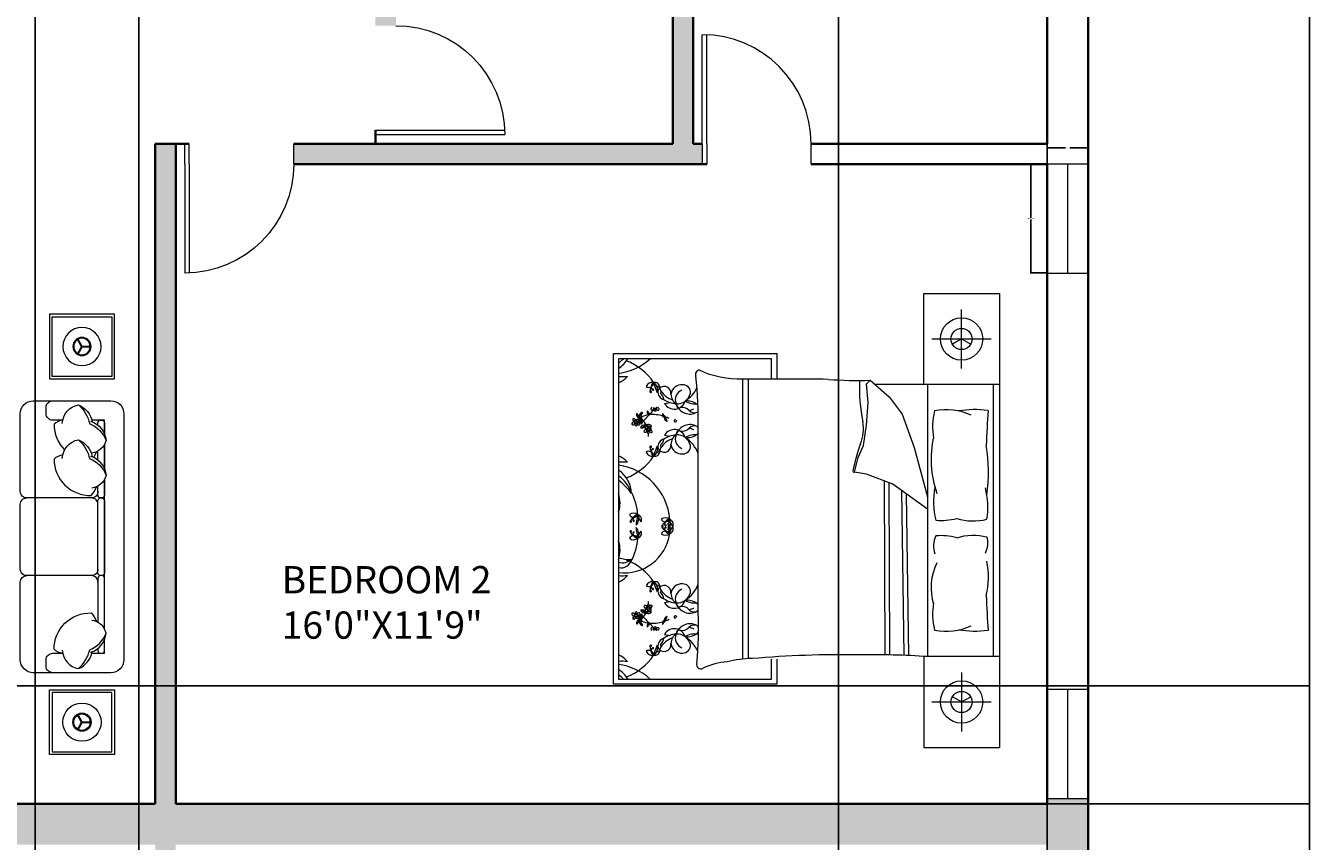
# Model space of a CAD drawing. Units: inches. Extents: x -26 to 13070, y -956 to 6917.
# Tile 9 of 13: x 314 to 597, y -466 to -286. Entities that reach past the tile are written whole.
import ezdxf

# ---------------------------------------------------------------- set-up
doc = ezdxf.new("R2010")
doc.units = ezdxf.units.IN
doc.header["$MEASUREMENT"] = 0
for name, color, linetype, lineweight in [('A-ANNO-DIMS', 2, 'Continuous', 18), ('A-AREA-IDEN', 7, 'Continuous', 18), ('A-DOOR', 3, 'Continuous', 18), ('A-FURN', 8, 'Continuous', 13), ('A-GLAZ', 4, 'Continuous', 18), ('A-WALL', 7, 'Continuous', 35), ('A-WALL-PATT', 252, 'Continuous', 13)]:
    doc.layers.add(name, color=color, linetype=linetype, lineweight=lineweight)
doc.styles.get("Standard").update_dxf_attribs({"font": 'arial.ttf'})
doc.dimstyles.get("Standard").update_dxf_attribs({"dimtxt": 0.18, "dimasz": 0.18, "dimexe": 0.18, "dimexo": 0.0625, "dimgap": 0.09, "dimtad": 0, "dimtih": 1, "dimtoh": 1, "dimdec": 0, "dimzin": 0, "dimdsep": 46, "dimlunit": 3, "dimtxsty": 'Standard', "dimcen": 0.09, "dimadec": 0, "dimazin": 0, "dimtfac": 1, "dimtdec": 0, "dimtofl": 0, "dimtmove": 0, "dimatfit": 3, "dimfxl": 1, "dimtolj": 1, "dimtzin": 0, "dimarcsym": 0})

# ---------------------------------------------------------------- blocks, each defined once
blk = doc.blocks.new('LIVING-END-TABLE')
for p, q in [((7.06, 7.09), (6.05, 8.83)), ((7.21, 7.18), (6.21, 8.92)), ((7.06, 7.18), (6.05, 5.44)), ((7.21, 7.09), (6.21, 5.35)), ((7.13, 7.22), (9.15, 7.22)), ((7.13, 7.04), (9.15, 7.04))]:
    blk.add_line(p, q)
at = {"ltscale": 0.03}
blk.add_lwpolyline([(0, 0), (0, 14.27), (14.27, 14.27), (14.27, 0)], close=True, dxfattribs=at)
blk.add_lwpolyline([(0.57, 13.7), (0.57, 0.57), (13.7, 0.57), (13.7, 13.7)], close=True)
for radius in [4.21, 2.01, 1.81]:
    blk.add_circle((7.13, 7.13), radius)
blk = doc.blocks.new('DOOR-SWING-24')
for p, q in [((24, 1), (0, 1)), ((24, 0), (0, 0))]:
    blk.add_line(p, q)
blk.add_arc((24, 0), 24, 90, 180)
blk = doc.blocks.new('WIN-24')
for p, q in [((0, 24), (0, 0)), ((9, 24), (0, 24)), ((4.5, 24), (4.5, 0)), ((9, 0), (9, 24)), ((0, 0), (9, 0))]:
    blk.add_line(p, q)
blk = doc.blocks.new('*D22')
at = {"layer": 'A-ANNO-DIMS', "color": 0, "lineweight": -2, "transparency": 16777216}
for p, q in [((538.58, -316.54), (534.86, -316.54)), ((535.04, -316.72), (535.04, -328.36)), ((535.04, -340.36), (535.04, -328.72)), ((538.58, -340.54), (534.86, -340.54))]:
    blk.add_line(p, q, dxfattribs=at)
at = {"layer": 'A-ANNO-DIMS', "color": 0, "transparency": 16777216}
for points in [[(535.01, -316.72), (535.07, -316.72), (535.04, -316.54)], [(535.01, -340.36), (535.07, -340.36), (535.04, -340.54)]]:
    blk.add_solid(points, dxfattribs=at)
at = {"layer": 'Defpoints', "color": 0, "transparency": 16777216}
for p in [(535.04, -316.54), (538.64, -316.54), (538.64, -340.54)]:
    blk.add_point(p, dxfattribs=at)
at = {"layer": 'A-ANNO-DIMS', "color": 0, "transparency": 16777216, "insert": (535.04, -328.54), "char_height": 0.18, "attachment_point": 5}
blk.add_mtext('\\A1;WINDOW 24 TYP.', dxfattribs=at)
blk = doc.blocks.new('*D23')
at = {"layer": 'A-ANNO-DIMS', "color": 0, "lineweight": -2, "transparency": 16777216}
for p, q in [((538.64, -316.48), (538.64, -312.76)), ((538.82, -312.94), (542.68, -312.94)), ((547.46, -312.94), (543.6, -312.94)), ((547.64, -316.48), (547.64, -312.76))]:
    blk.add_line(p, q, dxfattribs=at)
at = {"layer": 'A-ANNO-DIMS', "color": 0, "transparency": 16777216}
for points in [[(538.82, -312.91), (538.82, -312.97), (538.64, -312.94)], [(547.46, -312.91), (547.46, -312.97), (547.64, -312.94)]]:
    blk.add_solid(points, dxfattribs=at)
at = {"layer": 'Defpoints', "color": 0, "transparency": 16777216}
for p in [(547.64, -312.94), (538.64, -316.54), (547.64, -316.54)]:
    blk.add_point(p, dxfattribs=at)
at = {"layer": 'A-ANNO-DIMS', "color": 0, "transparency": 16777216, "insert": (543.14, -312.94), "char_height": 0.18, "attachment_point": 5}
blk.add_mtext('\\A1;9 TYP.', dxfattribs=at)
blk = doc.blocks.new('*D45')
at = {"layer": 'A-ANNO-DIMS', "color": 0, "lineweight": -2, "transparency": 16777216}
for p, q in [((547.7, 10.46), (596.57, 10.46)), ((596.39, 10.28), (596.39, -223.36)), ((596.39, -457.36), (596.39, -223.72)), ((538.7, -457.54), (596.57, -457.54))]:
    blk.add_line(p, q, dxfattribs=at)
at = {"layer": 'A-ANNO-DIMS', "color": 0, "transparency": 16777216}
for points in [[(596.36, 10.28), (596.42, 10.28), (596.39, 10.46)], [(596.36, -457.36), (596.42, -457.36), (596.39, -457.54)]]:
    blk.add_solid(points, dxfattribs=at)
at = {"layer": 'Defpoints', "color": 0, "transparency": 16777216}
for p in [(547.64, 10.46), (596.39, 10.46), (538.64, -457.54)]:
    blk.add_point(p, dxfattribs=at)
at = {"layer": 'A-ANNO-DIMS', "color": 0, "transparency": 16777216, "insert": (596.39, -223.54), "char_height": 0.18, "attachment_point": 5}
blk.add_mtext('\\A1;468', dxfattribs=at)
blk = doc.blocks.new('*D46')
at = {"layer": 'A-ANNO-DIMS', "color": 0, "lineweight": -2, "transparency": 16777216}
for p, q in [((538.7, -457.54), (596.57, -457.54)), ((596.39, -457.72), (596.39, -665.86)), ((596.39, -874.36), (596.39, -666.22)), ((547.7, -874.54), (596.57, -874.54))]:
    blk.add_line(p, q, dxfattribs=at)
at = {"layer": 'A-ANNO-DIMS', "color": 0, "transparency": 16777216}
for points in [[(596.36, -457.72), (596.42, -457.72), (596.39, -457.54)], [(596.36, -874.36), (596.42, -874.36), (596.39, -874.54)]]:
    blk.add_solid(points, dxfattribs=at)
at = {"layer": 'Defpoints', "color": 0, "transparency": 16777216}
for p in [(538.64, -457.54), (596.39, -457.54), (547.64, -874.54)]:
    blk.add_point(p, dxfattribs=at)
at = {"layer": 'A-ANNO-DIMS', "color": 0, "transparency": 16777216, "insert": (596.39, -666.04), "char_height": 0.18, "attachment_point": 5}
blk.add_mtext('\\A1;417', dxfattribs=at)
blk = doc.blocks.new('*D50')
at = {"layer": 'A-ANNO-DIMS', "color": 0, "lineweight": -2, "transparency": 16777216}
for p, q in [((315.7, -495.61), (315.7, 116.39)), ((315.88, 116.21), (326.72, 116.21)), ((338.35, 116.21), (327.51, 116.21)), ((338.53, -495.61), (338.53, 116.39))]:
    blk.add_line(p, q, dxfattribs=at)
at = {"layer": 'A-ANNO-DIMS', "color": 0, "transparency": 16777216}
for points in [[(315.88, 116.24), (315.88, 116.18), (315.7, 116.21)], [(338.35, 116.24), (338.35, 116.18), (338.53, 116.21)]]:
    blk.add_solid(points, dxfattribs=at)
at = {"layer": 'Defpoints', "color": 0, "transparency": 16777216}
for p in [(338.53, 116.21), (315.7, -495.67), (338.53, -495.67)]:
    blk.add_point(p, dxfattribs=at)
at = {"layer": 'A-ANNO-DIMS', "color": 0, "transparency": 16777216, "insert": (327.12, 116.21), "char_height": 0.18, "attachment_point": 5}
blk.add_mtext('\\A1;22.83', dxfattribs=at)
blk = doc.blocks.new('*D53')
at = {"layer": 'A-ANNO-DIMS', "color": 0, "lineweight": -2, "transparency": 16777216}
for p, q in [((492.64, -622.48), (492.64, 116.39)), ((492.82, 116.21), (515.42, 116.21)), ((538.46, 116.21), (515.86, 116.21)), ((538.64, -622.48), (538.64, 116.39))]:
    blk.add_line(p, q, dxfattribs=at)
at = {"layer": 'A-ANNO-DIMS', "color": 0, "transparency": 16777216}
for points in [[(492.82, 116.24), (492.82, 116.18), (492.64, 116.21)], [(538.46, 116.24), (538.46, 116.18), (538.64, 116.21)]]:
    blk.add_solid(points, dxfattribs=at)
at = {"layer": 'Defpoints', "color": 0, "transparency": 16777216}
for p in [(538.64, 116.21), (492.64, -622.54), (538.64, -622.54)]:
    blk.add_point(p, dxfattribs=at)
at = {"layer": 'A-ANNO-DIMS', "color": 0, "transparency": 16777216, "insert": (515.64, 116.21), "char_height": 0.18, "attachment_point": 5}
blk.add_mtext('\\A1;46', dxfattribs=at)
blk = doc.blocks.new('*D57')
at = {"layer": 'A-ANNO-DIMS', "color": 0, "lineweight": -2, "transparency": 16777216}
for p, q in [((154.7, -271.54), (596.57, -271.54)), ((596.39, -271.72), (596.39, -351.36)), ((596.39, -431.36), (596.39, -351.72)), ((154.7, -431.54), (596.57, -431.54))]:
    blk.add_line(p, q, dxfattribs=at)
at = {"layer": 'A-ANNO-DIMS', "color": 0, "transparency": 16777216}
for points in [[(596.36, -271.72), (596.42, -271.72), (596.39, -271.54)], [(596.36, -431.36), (596.42, -431.36), (596.39, -431.54)]]:
    blk.add_solid(points, dxfattribs=at)
at = {"layer": 'Defpoints', "color": 0, "transparency": 16777216}
for p in [(154.64, -271.54), (596.39, -271.54), (154.64, -431.54)]:
    blk.add_point(p, dxfattribs=at)
at = {"layer": 'A-ANNO-DIMS', "color": 0, "transparency": 16777216, "insert": (596.39, -351.54), "char_height": 0.18, "attachment_point": 5}
blk.add_mtext('\\A1;160', dxfattribs=at)

msp = doc.modelspace()

# ---------------------------------------------------------------- hatches: boundary and pattern name
at = {"layer": 'A-WALL-PATT'}
h = msp.add_hatch(color=256, dxfattribs=at)
h.dxf.hatch_style = 1
h.paths.add_polyline_path([(223.641, 10.458), (214.641, 10.458), (22.641, 10.458), (22.641, -171.042), (31.641, -171.042), (31.641, -135.042), (205.641, -135.042), (205.641, -241.042), (210.141, -241.042), (210.141, -130.542), (94.641, -130.542), (94.641, -76.542), (85.641, -76.542), (85.641, -126.042), (27.141, -126.042), (27.141, 5.958), (85.641, 5.958), (85.641, -52.542), (94.641, -52.542), (94.641, 1.458), (214.641, 1.458), (214.641, -16.542), (223.641, -16.542), (229.641, -16.542), (229.641, -7.542), (223.641, -7.542)])
h.paths.add_polyline_path([(367.048, 10.458), (346.641, 10.458), (337.641, 10.458), (337.641, -7.542), (331.641, -7.542), (331.641, -16.542), (337.641, -16.542), (342.141, -16.542), (342.141, -128.542), (346.641, -128.542), (346.641, 1.458), (367.048, 1.458)])
h.paths.add_polyline_path([(547.641, 10.458), (403.048, 10.458), (403.048, 1.458), (538.641, 1.458), (538.641, -46.542), (547.641, -46.542)])
h.paths.add_polyline_path([(547.641, -106.542), (538.641, -106.542), (538.641, -154.542), (481.013, -154.542), (481.013, -159.042), (538.641, -159.042), (547.641, -159.042)])
h.paths.add_polyline_path([(457.013, -154.542), (342.141, -154.542), (342.141, -165.042), (346.641, -165.042), (346.641, -159.042), (414.141, -159.042), (414.141, -225.042), (346.641, -225.042), (346.641, -189.042), (342.141, -189.042), (342.141, -234.042), (390.641, -234.042), (390.641, -286.042), (395.141, -286.042), (395.141, -234.042), (456.141, -234.042), (456.141, -312.042), (372.641, -312.042), (372.641, -316.542), (462.641, -316.542), (462.641, -312.042), (460.641, -312.042), (460.641, -234.042), (538.641, -234.042), (547.641, -234.042), (547.641, -195.042), (538.641, -195.042), (538.641, -225.042), (418.641, -225.042), (418.641, -159.042), (457.013, -159.042)])
h.paths.add_polyline_path([(547.641, -270.042), (538.641, -270.042), (538.641, -312.042), (486.641, -312.042), (486.641, -316.542), (538.641, -316.542), (547.641, -316.542)], flags=0)
h.paths.add_polyline_path([(547.641, -456.306), (538.641, -456.306), (538.641, -457.542), (346.641, -457.542), (346.641, -316.542), (346.641, -312.042), (342.141, -312.042), (342.141, -457.542), (145.641, -457.542), (145.641, -466.542), (342.141, -466.542), (342.141, -627.042), (346.641, -627.042), (346.641, -466.542), (538.641, -466.542), (538.641, -514.542), (547.641, -514.542)])
h.paths.add_polyline_path([(466.641, -622.542), (372.641, -622.542), (372.641, -627.042), (388.641, -627.042), (388.641, -721.542), (393.141, -721.542), (393.141, -627.042), (462.141, -627.042), (462.141, -717.042), (466.641, -717.042)])
h.paths.add_polyline_path([(547.641, -574.542), (538.641, -574.542), (538.641, -622.542), (492.641, -622.542), (492.641, -627.042), (538.641, -627.042), (538.641, -654.042), (547.641, -654.042)])
h.paths.add_polyline_path([(547.641, -690.042), (538.641, -690.042), (538.641, -717.042), (466.641, -717.042), (466.641, -721.542), (538.641, -721.542), (538.641, -763.542), (547.641, -763.542)])
h.paths.add_polyline_path([(462.141, -717.042), (419.141, -717.042), (419.141, -721.542), (462.141, -721.542)], flags=0)
h.paths.add_polyline_path([(346.641, -721.542), (352.641, -721.542), (352.641, -717.042), (342.141, -717.042), (342.141, -874.542), (342.141, -907.542), (351.141, -907.542), (351.141, -874.542), (395.949, -874.542), (395.949, -865.542), (351.141, -865.542), (351.141, -841.542), (346.641, -841.542)])
h.paths.add_polyline_path([(547.641, -823.542), (538.641, -823.542), (538.641, -865.542), (431.949, -865.542), (431.949, -874.542), (547.641, -874.542)])
h.paths.add_polyline_path([(172.641, -865.713), (140.641, -865.744), (140.641, -788.744), (182.646, -788.704), (182.641, -784.204), (136.141, -784.249), (136.141, -848.332), (131.641, -848.332), (131.641, -874.542), (172.641, -874.542)])
h.paths.add_polyline_path([(217.641, -816.13), (213.141, -816.13), (213.141, -784.174), (208.641, -784.179), (208.641, -865.679), (208.641, -874.542), (217.641, -874.542)])
h.paths.add_polyline_path([(95.641, -865.788), (31.641, -865.849), (31.641, -832.695), (22.641, -832.695), (22.641, -874.542), (95.641, -874.542)])
h.paths.add_polyline_path([(217.641, -741.17), (31.641, -741.349), (31.641, -708.349), (22.641, -708.349), (22.641, -772.542), (22.641, -796.695), (31.641, -796.695), (31.641, -763.542), (31.641, -745.849), (217.641, -745.67)])
h.paths.add_polyline_path([(31.641, -651.349), (99.65, -651.284), (99.641, -642.284), (31.641, -642.349), (31.641, -639.042), (31.641, -588.349), (125.641, -588.259), (125.641, -651.259), (134.641, -651.25), (134.641, -579.25), (112.641, -579.271), (112.641, -549.042), (112.641, -504.271), (85.633, -504.297), (85.641, -513.297), (103.641, -513.28), (103.641, -549.042), (103.641, -579.28), (31.641, -579.349), (31.641, -549.042), (31.641, -513.349), (49.641, -513.314), (49.633, -504.332), (31.641, -504.349), (22.641, -504.358), (22.641, -684.349), (31.641, -684.349)])
h.paths.add_polyline_path([(31.641, -276.042), (145.641, -276.042), (145.641, -402.042), (145.641, -419.542), (154.641, -419.542), (154.641, -411.042), (154.641, -271.542), (210.141, -271.542), (210.141, -265.042), (205.641, -265.042), (205.641, -267.042), (31.641, -267.042), (31.641, -231.042), (22.641, -231.042), (22.641, -426.852), (31.641, -426.852), (31.641, -411.042), (31.641, -402.042)])

# ---------------------------------------------------------------- linework, layer by layer
at = {"layer": 'A-DOOR'}
for p, q in [((390.641, -309.042), (395.141, -309.042)), ((390.641, -310.042), (395.141, -310.042)), ((348.641, -316.542), (348.641, -312.042)), ((349.641, -316.542), (349.641, -312.042)), ((372.641, -316.542), (372.641, -312.042)), ((462.641, -312.042), (462.641, -316.542)), ((463.641, -312.042), (463.641, -316.542)), ((486.641, -316.542), (486.641, -312.042))]:
    msp.add_line(p, q, dxfattribs=at)
at = {"layer": 'A-FURN'}
for p, q in [((528.091, -345.081), (528.091, -445.074)), ((519.758, -361.613), (519.758, -348.547)), ((513.225, -355.08), (526.291, -355.08)), ((443.054, -358.279), (479.074, -358.279)), ((443.054, -431.178), (443.054, -358.279)), ((479.074, -358.279), (479.074, -363.935)), ((444.212, -359.438), (444.212, -430.019)), ((477.915, -359.438), (444.212, -359.438)), ((477.915, -363.933), (477.915, -359.438)), ((471.59, -425.624), (471.59, -363.927)), ((472.837, -425.529), (472.837, -363.927)), ((498.792, -364.994), (499.602, -364.184)), ((499.197, -369.045), (498.792, -364.994)), ((499.602, -364.184), (503.852, -367.83)), ((528.091, -365.08), (500.645, -365.08)), ((503.852, -367.83), (506.686, -371.678)), ((512.289, -365.08), (512.289, -425.075)), ((526.807, -425.075), (526.807, -365.08)), ((454.35, -369.292), (455.48, -369.07)), ((498.792, -374.108), (499.197, -369.045)), ((506.686, -371.678), (509.317, -378.969)), ((454.35, -376.28), (455.48, -376.501)), ((461.768, -415.377), (461.768, -374.778)), ((498.185, -378.564), (498.792, -374.108)), ((496.97, -381.197), (498.185, -378.564)), ((509.317, -378.969), (512.289, -389.873)), ((496.161, -384.437), (496.97, -381.197)), ((498.792, -384.842), (496.161, -384.437)), ((504.662, -387.07), (498.792, -384.842)), ((502.934, -424.721), (502.776, -386.354)), ((503.96, -424.716), (503.809, -386.747)), ((512.289, -392.549), (504.662, -387.07)), ((507.109, -424.768), (506.596, -388.46)), ((508.135, -424.807), (507.636, -389.207)), ((454.35, -413.177), (455.48, -412.956)), ((454.35, -420.165), (455.48, -420.387)), ((477.915, -430.019), (477.915, -425.612)), ((479.074, -425.633), (479.074, -431.178)), ((444.212, -430.019), (477.915, -430.019)), ((519.758, -428.542), (519.758, -441.607)), ((479.074, -431.178), (443.054, -431.178)), ((513.225, -435.074), (526.291, -435.074))]:
    msp.add_line(p, q, dxfattribs=at)
for points in [[(511.425, -365.08), (511.425, -345.081), (528.091, -345.081)], [(519.758, -355.08), (517.737, -356.247)], [(519.758, -355.08), (521.778, -356.247)], [(330.949, -383.667), (330.949, -378.353)], [(330.949, -418.973), (330.949, -386.04)], [(328.145, -424.349), (330.949, -424.349), (330.949, -421.347)], [(528.091, -425.075), (511.425, -425.075), (511.425, -445.074), (528.091, -445.074)], [(519.758, -435.074), (517.737, -433.908)], [(519.758, -435.074), (521.778, -433.908)]]:
    msp.add_lwpolyline(points, dxfattribs=at)
for points in [[(490.446, -363.975, 0.0012423), (471.473, -363.927, -0.1272016), (462.018, -361.923)], [(321.744, -372.977), (319.533, -372.977, -0.4142136), (318.106, -371.551), (318.106, -370.124, -0.4142136), (319.533, -368.697)], [(321.658, -373.694, -0.3567724), (325.255, -369.605, -0.2495421), (328.219, -373.31, 9.6168803)], [(325.255, -369.605, -0.1477299), (327.707, -373.775, -0.2133428), (331.304, -377.455, -0.1786618)], [(525.598, -370.823, 0.0748968), (519.067, -370.944, -0.4728166)], [(321.745, -372.974, 0.1655406), (319.859, -373.857, 0.2002311), (322.156, -379.522, 0.1215233)], [(327.903, -373.199, -0.3066635), (331.304, -377.455, -0.30633), (328.198, -380.236, 0.8728472)], [(330.949, -375.979), (330.949, -372.977), (328.145, -372.977, -0.4142136)], [(329.522, -374.066), (329.522, -373.548, -0.4142136), (330.093, -372.977), (330.378, -372.977, -0.4142136), (330.949, -373.548)], [(330.949, -373.548), (330.949, -375.979, -0.4142136)], [(321.658, -381.381, -0.3567724), (325.255, -377.292, -0.2495421), (328.219, -380.997, 9.6168803)], [(325.255, -377.292, -0.1477299), (327.707, -381.462, -0.2133428), (331.304, -385.142, -0.1786618)], [(330.949, -378.353), (330.949, -383.667, -0.4142136)], [(321.745, -380.661, 0.1655406), (319.859, -381.544, 0.4259892), (328.034, -389.558, 0.1215233), (329.161, -387.656, -7.1154643)], [(327.903, -380.886, -0.3066635), (331.304, -385.142, -0.30633), (328.198, -387.923, 0.8728472)], [(328.603, -381.165, 0.0718654), (329.161, -379.969, -7.1154643)], [(329.522, -381.754), (329.522, -379.79, -0.4142136)], [(330.949, -386.04), (330.949, -389.53, -0.4142136), (330.378, -390.101), (330.093, -390.101, -0.4142136), (329.522, -389.53), (329.522, -387.477, -0.4142136)], [(329.522, -388.674, -0.4142136), (328.095, -390.101), (313.825, -390.101, -0.4142136)], [(329.522, -391.528, 0.4142136), (328.095, -390.101)], [(518.702, -394.609, 0.1409896), (525.365, -394.809, 0.2352448)], [(518.702, -398.879, -0.1409896), (525.365, -398.679, -0.2352448)], [(329.522, -408.652, 0.4142136), (328.095, -407.225), (313.825, -407.225, 0.4142136)], [(329.522, -405.798, -0.4142136), (328.095, -407.225)], [(330.949, -418.973), (330.949, -407.796, 0.4142136), (330.378, -407.225), (330.093, -407.225, 0.4142136), (329.522, -407.796), (329.522, -417.536, 0.4142136)], [(321.745, -424.352, -0.1655406), (319.859, -423.469, -0.4259892), (328.034, -415.455, -0.1215233), (329.161, -417.357, 7.1154643)], [(327.903, -424.127, 0.3066635), (331.304, -419.871, 0.30633), (328.198, -417.09, -0.8728472)], [(325.255, -427.721, 0.1477299), (327.707, -423.551, 0.2133428), (331.304, -419.871, 0.1786618)], [(330.949, -423.778), (330.949, -421.347, 0.4142136)], [(525.598, -419.332, -0.0748968), (519.067, -419.211, 0.4728166)], [(319.533, -428.63, -0.4142136), (318.106, -427.203), (318.106, -425.776, -0.4142136), (319.533, -424.349), (321.744, -424.349)], [(321.658, -423.633, 0.3567724), (325.255, -427.721, 0.2495421), (328.219, -424.016, -9.6168803)], [(329.522, -423.26), (329.522, -423.778, 0.4142136), (330.093, -424.349), (330.378, -424.349, 0.4142136), (330.949, -423.778)], [(473.625, -425.502, 0.0561118), (468.123, -426.227, 0.0953413), (462.824, -427.633)]]:
    msp.add_lwpolyline(points, format="xyb", dxfattribs=at)
at = {"layer": 'A-FURN', "ltscale": 0.03}
msp.add_lwpolyline([(315.252, -428.63, -0.4142136), (312.398, -425.776), (312.398, -408.652, -0.4142136), (313.825, -407.225, -0.4142136), (312.398, -405.798), (312.398, -391.528, -0.4142136), (313.825, -390.101, -0.4142136), (312.398, -388.674), (312.398, -371.551, -0.4142136), (315.252, -368.697), (332.376, -368.697, -0.4142136), (335.23, -371.551), (335.23, -425.776, -0.4142136), (332.376, -428.63)], format="xyb", close=True, dxfattribs=at)
at = {"layer": 'A-FURN'}
msp.add_lwpolyline([(330.949, -390.672), (330.949, -406.654, -0.4142136), (330.378, -407.225), (330.093, -407.225, -0.4142136), (329.522, -406.654), (329.522, -390.672, -0.4142136), (330.093, -390.101), (330.378, -390.101, -0.4142136)], format="xyb", close=True, dxfattribs=at)
for centre, radius in [((519.758, -355.08), 4.666), ((519.758, -355.08), 2.333), ((448.042, -373.403), 0.255), ((450.727, -375.068), 0.255), ((448.042, -416.054), 0.255), ((450.727, -414.389), 0.255), ((519.758, -435.074), 4.666), ((519.758, -435.074), 2.333)]:
    msp.add_circle(centre, radius, dxfattribs=at)
for centre, radius, start, end in [((439.518, -353.978), 7.929, 306.30357, 316.48142), ((440.704, -356.267), 6.363, 303.46172, 330.11157), ((442.453, -349.717), 13.058, 277.74496, 311.8856), ((441.162, -372.056), 13.058, 34.38655, 68.59079), ((462.082, -362.843), 0.923, 93.97998, 207.34124), ((442.176, -359.831), 5.309, 292.55474, 318.95456), ((445.029, -345.288), 18.066, 267.40811, 273.65191), ((451.629, -366.096), 1.448, 77.71153, 159.03868), ((450.847, -364.649), 1.09, 238.46331, 358.28689), ((454.424, -366.855), 3.302, 138.84017, 177.9352), ((452.434, -365.627), 1.068, 117.6827, 223.77619), ((452.194, -365.733), 1.082, 2.95159, 103.72796), ((460.855, -362.702), 9.135, 192.51726, 207.18239), ((450.731, -366.357), 2.064, 345.46535, 54.23429), ((453.841, -363.52), 2.23, 211.38267, 255.29688), ((357.682, -373.585), 104.093, 359.34325, 5.68869), ((497.116, -272.501), 91.717, 265.82941, 271.55305), ((535.011, -365.896), 37.739, 177.45188, 191.3392), ((451.286, -366.742), 0.162, 177.9352, 11.4834), ((451.367, -366.725), 0.0788, 11.4834, 127.94089), ((451.764, -366.269), 0.141, 223.77619, 159.71835), ((454.72, -366.644), 1.874, 175.96902, 254.3045), ((454.269, -367.004), 1.501, 350.26398, 160.86884), ((452.643, -366.695), 0.92, 333.97555, 53.26805), ((452.229, -368.663), 1.996, 6.1662, 51.58255), ((457.572, -364.029), 4.721, 211.26137, 251.7045), ((458.119, -367.554), 2.39, 84.94485, 172.88575), ((458.65, -367.139), 2.905, 182.3591, 234.04014), ((459.025, -368.493), 2.32, 111.58187, 201.42215), ((457.111, -366.344), 3.007, 265.29334, 346.921), ((458.36, -366.862), 1.688, 354.48557, 91.05378), ((454.726, -362.453), 7.568, 303.66712, 333.29966), ((444.529, -364.814), 9.494, 313.15413, 322.0459), ((451.511, -370.518), 0.195, 142.47371, 265.05304), ((451.768, -370.479), 0.42, 127.76209, 169.04026), ((451.545, -370.123), 0.592, 265.05304, 338.36176), ((452.328, -370.933), 0.773, 113.42757, 137.61037), ((452.24, -370.132), 0.255, 183.27684, 356.72316), ((452.427, -370.592), 0.417, 139.78892, 227.67915), ((451.444, -370.587), 0.834, 353.08516, 15.71709), ((451.992, -370.687), 0.526, 350.3487, 43.65382), ((452.967, -370.143), 0.612, 198.72627, 262.50315), ((452.481, -370.429), 0.243, 1.10805, 91.86747), ((452.937, -370.56), 0.197, 255.23556, 54.9248), ((452.634, -370.484), 0.425, 11.56373, 52.6358), ((457.191, -363.985), 5.366, 236.28828, 266.5076), ((456.505, -368.052), 2.486, 209.90854, 343.1337), ((457.55, -369.626), 0.621, 167.30406, 285.14713), ((459.23, -372.596), 3.856, 122.70113, 126.34448), ((459.952, -368.437), 3.187, 199.28218, 299.1751), ((458.247, -372.204), 2.05, 41.56531, 105.14713), ((461.028, -365.229), 4.143, 238.82178, 279.15542), ((459.23, -372.596), 3.856, 55.78505, 94.73037), ((459.375, -367.956), 2.874, 277.43599, 299.91487), ((460.662, -370.36), 1.204, 30.0293, 52.32497), ((516.445, -383.562), 12.888, 65.1316, 101.75834), ((447.571, -373.75), 0.42, 61.21959, 169.04026), ((447.848, -372.884), 0.503, 157.40857, 261.43859), ((447.564, -372.868), 0.252, 58.0499, 135.62681), ((448.131, -374.204), 0.773, 113.42757, 137.61037), ((447.828, -373.026), 0.169, 172.90601, 277.13198), ((447.273, -373.335), 0.803, 14.75581, 58.0499), ((448.397, -373.122), 0.347, 36.10456, 181.42811), ((448.414, -371.76), 0.284, 124.3538, 214.39233), ((448.831, -371.802), 0.663, 190.30568, 287.1958), ((448.194, -372.848), 0.351, 270.06451, 331.15075), ((448.493, -372.932), 0.4, 221.84125, 265.78771), ((449.022, -371.566), 0.77, 176.97007, 248.29129), ((454.515, -367.509), 7.439, 212.6784, 216.37461), ((448.283, -373.7), 0.243, 1.10805, 91.86747), ((448.491, -373.083), 0.249, 263.75256, 41.70535), ((448.437, -373.755), 0.425, 11.56373, 86.36503), ((448.762, -371.746), 0.294, 216.37461, 291.75478), ((451.367, -375.878), 4.152, 124.00334, 132.49171), ((447.097, -376.402), 4.435, 63.78194, 68.29129), ((449.465, -372.989), 0.706, 128.32082, 208.81623), ((449.465, -371.952), 0.663, 122.81548, 187.39917), ((449.593, -372.937), 0.843, 207.70426, 254.35163), ((448.954, -372.226), 0.222, 289.36054, 111.75478), ((449.12, -372.227), 0.222, 221.87034, 44.26458), ((450.126, -372.872), 1.161, 157.23048, 229.06353), ((449.756, -372.037), 0.77, 109.47987, 177.68284), ((449.736, -372.489), 0.683, 174.45436, 220.61881), ((445.852, -376.305), 4.98, 30.54402, 49.81798), ((449.344, -371.55), 0.284, 56.86359, 146.90213), ((449.49, -371.867), 0.294, 148.88441, 224.26458), ((448.594, -373.468), 0.821, 340.00407, 40.61881), ((455.607, -375.559), 7.439, 145.1882, 148.88441), ((451.367, -375.878), 4.152, 94.75602, 119.20408), ((460.207, -381.855), 13.663, 132.24124, 142.17444), ((453.31, -370.981), 2.82, 178.32639, 187.13024), ((450.265, -371.373), 0.525, 11.32561, 64.46214), ((452.046, -370.618), 1.58, 190.25878, 210.65599), ((450.986, -371.262), 0.48, 188.34322, 274.28685), ((451.408, -370.996), 0.838, 210.65599, 242.63414), ((452.042, -370.276), 1.607, 218.21012, 226.30712), ((450.854, -371.626), 0.204, 325.76575, 67.44165), ((451.575, -380.004), 8.282, 73.58418, 93.82768), ((452.294, -370.738), 0.219, 227.67915, 350.3487), ((456.674, -371.577), 2.82, 178.32639, 187.13024), ((453.629, -371.968), 0.525, 11.32561, 64.46214), ((455.411, -371.213), 1.58, 190.25878, 210.65599), ((454.351, -371.857), 0.48, 188.34322, 274.28685), ((454.772, -371.592), 0.838, 210.65599, 242.63414), ((455.406, -370.872), 1.607, 218.21012, 226.30712), ((454.218, -372.221), 0.204, 325.76575, 67.44165), ((454.792, -372.594), 0.48, 147.53317, 233.47681), ((454.408, -372.539), 0.204, 354.37838, 96.05427), ((455.225, -372.348), 0.838, 179.18588, 211.16403), ((451.575, -380.004), 8.282, 63.0032, 69.89408), ((456.136, -370.678), 2.82, 234.68979, 243.49364), ((455.86, -371.964), 1.58, 211.16403, 231.56124), ((456.159, -372.129), 1.607, 195.51291, 203.60991), ((454.353, -373.177), 0.525, 357.35788, 50.49441), ((456.608, -373.073), 0.193, 12.70507, 190.43845), ((456.727, -373.051), 0.313, 190.43845, 10.41356), ((460.901, -369.851), 1.496, 221.56531, 293.83541), ((460.662, -370.36), 1.204, 314.45169, 333.55801), ((490.029, -374.916), 8.14, 336.26158, 11.3392), ((526.769, -374.39), 13.4, 165.10393, 191.03689), ((1477.198, -425.938), 953.194, 176.685209, 177.149775), ((447.313, -373.789), 0.195, 142.47371, 265.05304), ((447.347, -373.394), 0.592, 265.05304, 338.36176), ((448.23, -373.863), 0.417, 139.78892, 227.67915), ((448.097, -374.009), 0.219, 227.67915, 350.3487), ((447.247, -373.858), 0.834, 353.08516, 15.71709), ((447.794, -373.958), 0.526, 350.3487, 43.65382), ((448.77, -373.414), 0.612, 198.72627, 262.50315), ((448.74, -373.831), 0.197, 255.23556, 54.9248), ((449.044, -373.421), 1.161, 270.278, 342.11105), ((449.818, -374.871), 0.821, 98.72271, 159.33746), ((449.406, -373.817), 0.843, 244.9899, 291.63727), ((449.59, -373.384), 0.683, 278.72271, 324.88717), ((449.47, -373.94), 0.706, 290.5253, 358.5375), ((449.997, -375.454), 0.195, 142.47371, 265.05304), ((450.255, -375.415), 0.42, 61.21959, 169.04026), ((450.031, -375.059), 0.592, 265.05304, 338.36176), ((450.532, -374.55), 0.503, 157.40857, 261.43859), ((450.249, -374.533), 0.252, 58.0499, 135.62681), ((450.846, -373.739), 0.706, 182.84988, 266.12261), ((450.572, -373.24), 0.683, 231.76073, 277.92519), ((451.105, -373.119), 1.161, 214.53686, 286.36991), ((450.815, -375.869), 0.773, 113.42757, 137.61037), ((450.512, -374.691), 0.169, 172.90601, 277.13198), ((449.957, -375), 0.803, 14.75581, 58.0499), ((445.852, -376.305), 4.98, 23.05007, 23.84774), ((450.914, -375.529), 0.417, 139.78892, 227.67915), ((450.781, -375.675), 0.219, 227.67915, 350.3487), ((450.779, -374.73), 0.821, 37.31045, 97.92519), ((451.081, -374.787), 0.347, 36.10456, 181.42811), ((449.931, -375.524), 0.834, 353.08516, 15.71709), ((450.872, -373.603), 0.843, 265.01064, 311.65801), ((445.852, -376.305), 4.98, 357.10709, 4.75853), ((450.478, -375.623), 0.526, 350.3487, 43.65382), ((451.454, -375.08), 0.612, 198.72627, 262.50315), ((450.879, -374.514), 0.351, 270.06451, 331.15075), ((451.177, -374.597), 0.4, 221.84125, 265.78771), ((450.968, -375.365), 0.243, 1.10805, 91.86747), ((451.175, -374.749), 0.249, 263.75256, 41.70535), ((451.121, -375.421), 0.425, 11.56373, 86.36503), ((451.424, -375.496), 0.197, 255.23556, 54.9248), ((457.191, -381.587), 5.366, 93.4924, 123.71172), ((456.505, -377.519), 2.486, 16.8663, 150.09146), ((458.65, -378.433), 2.905, 125.95986, 177.6409), ((459.025, -377.078), 2.32, 158.57785, 248.41813), ((457.111, -379.228), 3.007, 13.079, 94.70666), ((457.55, -375.945), 0.621, 74.85287, 192.69594), ((459.952, -377.134), 3.187, 60.8249, 160.71782), ((459.23, -372.976), 3.856, 233.65552, 237.29887), ((458.247, -373.367), 2.05, 254.85287, 318.43469), ((461.028, -380.342), 4.143, 79.71335, 121.17822), ((459.23, -372.976), 3.856, 265.26963, 304.21495), ((459.375, -377.615), 2.874, 60.08513, 82.56401), ((460.901, -375.72), 1.496, 66.16459, 138.43469), ((460.662, -375.211), 1.204, 307.67503, 336.71436), ((460.662, -375.211), 1.204, 23.22901, 45.54831), ((451.286, -378.829), 0.162, 348.5166, 182.0648), ((454.424, -378.716), 3.302, 182.0648, 221.15983), ((451.367, -378.846), 0.0788, 232.05911, 348.5166), ((452.434, -379.944), 1.068, 136.22381, 242.3173), ((450.731, -379.215), 2.064, 305.76571, 14.53465), ((460.855, -382.87), 9.135, 152.81761, 167.48274), ((454.72, -378.927), 1.874, 105.6955, 184.03098), ((454.269, -378.567), 1.501, 199.13116, 9.73602), ((452.643, -378.876), 0.92, 306.73195, 26.02445), ((452.229, -376.909), 1.996, 308.41745, 353.8338), ((457.572, -381.542), 4.721, 108.2955, 148.73863), ((458.119, -378.017), 2.39, 187.11425, 275.05515), ((458.36, -378.71), 1.688, 268.94622, 5.51443), ((454.726, -383.118), 7.568, 21.49413, 56.33288), ((533.947, -391.38), 38.778, 160.11942, 169.33829), ((536.294, -381.444), 23.242, 168.03974, 199.26152), ((489.415, -384.524), 36.265, 352.21958, 9.49698), ((442.176, -385.741), 5.309, 41.04544, 67.44526), ((441.162, -373.515), 13.058, 291.40921, 325.61345), ((450.847, -380.922), 1.09, 1.71311, 121.53669), ((451.629, -379.475), 1.448, 200.96132, 282.28847), ((451.818, -379.318), 0.0851, 200.26671, 136.22708), ((452.194, -379.838), 1.082, 256.27204, 357.04841), ((453.841, -382.051), 2.23, 104.70312, 148.61733), ((445.029, -400.284), 18.066, 86.34809, 92.59189), ((442.453, -395.855), 13.058, 4.46233, 82.25504), ((440.704, -389.304), 6.363, 1.27197, 56.53828), ((496.079, -384.21), 0.241, 178.86235, 289.75363), ((439.518, -391.593), 7.929, 17.85038, 53.69643), ((437.289, -395.76), 11.794, 34.01234, 54.05304), ((437.347, -391.203), 7.18, 343.54311, 17.0202), ((435.459, -394.855), 13.058, 4.46233, 27.4146), ((531.219, -390.853), 17.633, 169.86169, 193.62376), ((507.742, -392.183), 17.817, 351.52493, 13.95996), ((433.646, -394.048), 10.617, 4.37872, 5.63574), ((426.372, -399.64), 18.973, 19.72171, 19.90284), ((447.504, -394.912), 1.448, 47.78732, 129.11446), ((447.548, -393.267), 1.09, 208.5391, 328.36268), ((446.884, -395.3), 0.162, 148.01098, 341.55918), ((449.547, -396.963), 3.302, 108.91595, 148.01098), ((446.963, -395.326), 0.0788, 341.55918, 98.01668), ((448.435, -394.906), 1.068, 87.75849, 193.85198), ((447.535, -395.128), 0.141, 193.85198, 129.92454), ((457.193, -396.572), 9.135, 162.59304, 177.25817), ((446.595, -394.689), 2.064, 315.54113, 24.31008), ((450.706, -393.782), 2.23, 181.45846, 225.37266), ((448.175, -394.879), 1.082, 333.02737, 73.80375), ((454.498, -395.911), 1.448, 47.78732, 129.11446), ((454.542, -394.267), 1.09, 208.5391, 328.36268), ((456.541, -397.963), 3.302, 108.91595, 148.01098), ((455.429, -395.906), 1.068, 87.75849, 193.85198), ((454.529, -396.128), 0.141, 193.85198, 129.92454), ((453.589, -395.689), 2.064, 315.54113, 24.31008), ((464.187, -397.571), 9.135, 162.59304, 177.25817), ((453.589, -397.101), 2.064, 335.68992, 44.45887), ((464.187, -395.219), 9.135, 182.74183, 197.40696), ((455.169, -395.878), 1.082, 333.02737, 73.80375), ((457.7, -394.782), 2.23, 181.45846, 225.37266), ((515.36, -382.822), 12.252, 264.01289, 285.82928), ((445.468, -396.513), 10.106, 262.86355, 351.81966), ((447.548, -399.523), 1.09, 31.63732, 151.4609), ((447.504, -397.879), 1.448, 230.88554, 312.21268), ((446.884, -397.491), 0.162, 18.44082, 211.98902), ((449.547, -395.827), 3.302, 211.98902, 251.08405), ((446.963, -397.464), 0.0788, 261.98332, 18.44082), ((435.459, -397.935), 13.058, 332.5854, 355.53767), ((448.435, -397.884), 1.068, 166.14802, 272.24151), ((447.59, -397.648), 0.0851, 230.19092, 166.02088), ((457.193, -396.218), 9.135, 182.74183, 197.40696), ((446.595, -398.101), 2.064, 335.68992, 44.45887), ((450.706, -399.008), 2.23, 134.62734, 178.54154), ((448.175, -397.911), 1.082, 286.19625, 26.97263), ((454.542, -398.523), 1.09, 31.63732, 151.4609), ((454.498, -396.879), 1.448, 230.88554, 312.21268), ((453.878, -396.299), 0.162, 148.01098, 341.55918), ((453.878, -396.491), 0.162, 18.44082, 211.98902), ((456.541, -394.827), 3.302, 211.98902, 251.08405), ((453.957, -396.326), 0.0788, 341.55918, 98.01668), ((453.957, -396.464), 0.0788, 261.98332, 18.44082), ((455.429, -396.884), 1.068, 166.14802, 272.24151), ((454.583, -396.649), 0.0851, 230.19092, 166.02088), ((455.169, -396.912), 1.082, 286.19625, 26.97263), ((457.7, -398.008), 2.23, 134.62734, 178.54154), ((518.887, -400.72), 5.301, 155.01826, 198.54073), ((515.36, -410.666), 12.252, 74.17072, 95.98711), ((520.612, -400.051), 4.947, 333.34374, 16.10256), ((437.347, -401.587), 7.18, 342.9798, 16.45689), ((433.646, -398.742), 10.617, 354.36426, 355.62128), ((426.372, -393.15), 18.973, 340.09716, 340.27829), ((446.391, -397.82), 5.846, 248.11703, 276.61954), ((444.764, -403.183), 2.344, 256.38982, 349.07385), ((445.086, -401.421), 2.964, 252.86088, 311.90487), ((441.162, -415.942), 13.058, 34.38655, 68.59079), ((525.781, -409.982), 12.729, 153.87611, 196.17464), ((508.102, -407.464), 17.578, 346.34271, 11.1841), ((445.029, -389.173), 18.066, 267.40811, 273.65191), ((442.176, -403.716), 5.309, 292.55474, 318.95456), ((451.629, -409.982), 1.448, 77.71153, 159.03868), ((450.847, -408.535), 1.09, 238.46331, 358.28689), ((454.424, -410.741), 3.302, 138.84017, 177.9352), ((452.434, -409.513), 1.068, 117.6827, 223.77619), ((451.764, -410.154), 0.141, 223.77619, 159.71835), ((452.194, -409.619), 1.082, 2.95159, 103.72796), ((453.841, -407.406), 2.23, 211.38267, 255.29688), ((450.731, -410.242), 2.064, 345.46535, 54.23429), ((460.855, -406.587), 9.135, 192.51726, 207.18239), ((454.269, -410.89), 1.501, 350.26398, 160.86884), ((452.643, -410.581), 0.92, 333.97555, 53.26805), ((458.119, -411.44), 2.39, 84.94485, 172.88575), ((459.025, -412.379), 2.32, 111.58187, 201.42215), ((458.36, -410.747), 1.688, 354.48557, 91.05378), ((454.726, -406.339), 7.568, 303.66712, 338.50587), ((445.852, -413.152), 4.98, 355.24147, 2.89291), ((451.286, -410.627), 0.162, 177.9352, 11.4834), ((451.367, -410.611), 0.0788, 11.4834, 127.94089), ((454.72, -410.53), 1.874, 175.96902, 254.3045), ((452.229, -412.548), 1.996, 6.1662, 51.58255), ((457.572, -407.915), 4.721, 211.26137, 251.7045), ((457.191, -407.87), 5.366, 236.28828, 266.5076), ((456.505, -411.938), 2.486, 209.90854, 343.1337), ((458.65, -411.024), 2.905, 182.3591, 234.04014), ((457.111, -410.229), 3.007, 265.29334, 346.921), ((461.028, -409.114), 4.143, 238.82178, 280.28665), ((459.23, -416.481), 3.856, 55.78505, 94.73037), ((1477.198, -364.217), 953.194, 182.850225, 183.314791), ((447.313, -415.668), 0.195, 94.94696, 217.52629), ((447.571, -415.707), 0.42, 190.95974, 298.78041), ((447.347, -416.063), 0.592, 21.63824, 94.94696), ((448.131, -415.253), 0.773, 222.38963, 246.57243), ((448.23, -415.593), 0.417, 132.32085, 220.21108), ((448.097, -415.448), 0.219, 9.6513, 132.32085), ((447.247, -415.599), 0.834, 344.28291, 6.91484), ((447.794, -415.499), 0.526, 316.34618, 9.6513), ((448.77, -416.043), 0.612, 97.49685, 161.27373), ((448.283, -415.757), 0.243, 268.13253, 358.89195), ((448.437, -415.702), 0.425, 273.63497, 348.43627), ((448.74, -415.626), 0.197, 305.0752, 104.76444), ((449.593, -416.52), 0.843, 105.64837, 152.29574), ((450.126, -416.585), 1.161, 130.93647, 202.76952), ((449.406, -415.64), 0.843, 68.36273, 115.0101), ((449.044, -416.036), 1.161, 17.88895, 89.722), ((449.818, -414.586), 0.821, 200.66254, 261.27729), ((445.852, -413.152), 4.98, 310.18202, 329.45598), ((448.594, -415.989), 0.821, 319.38119, 19.99593), ((460.207, -407.602), 13.663, 217.82556, 227.75876), ((449.59, -416.073), 0.683, 35.11283, 81.27729), ((449.47, -415.517), 0.706, 1.4625, 69.4747), ((449.997, -414.003), 0.195, 94.94696, 217.52629), ((450.255, -414.042), 0.42, 190.95974, 298.78041), ((450.031, -414.398), 0.592, 21.63824, 94.94696), ((450.532, -414.907), 0.503, 98.56141, 202.59143), ((450.249, -414.924), 0.252, 224.37319, 301.9501), ((450.846, -415.718), 0.706, 93.87739, 177.15012), ((451.105, -416.338), 1.161, 73.63009, 145.46314), ((450.572, -416.216), 0.683, 82.07481, 128.23927), ((450.815, -413.588), 0.773, 222.38963, 246.57243), ((450.512, -414.766), 0.169, 82.86802, 187.09399), ((449.957, -414.457), 0.803, 301.9501, 345.24419), ((445.852, -413.152), 4.98, 336.15226, 336.94993), ((450.914, -413.928), 0.417, 132.32085, 220.21108), ((450.781, -413.782), 0.219, 9.6513, 132.32085), ((450.779, -414.727), 0.821, 262.07481, 322.68955), ((449.931, -413.933), 0.834, 344.28291, 6.91484), ((451.081, -414.67), 0.347, 178.57189, 323.89544), ((450.872, -415.854), 0.843, 48.34199, 94.98936), ((450.478, -413.833), 0.526, 316.34618, 9.6513), ((451.454, -414.377), 0.612, 97.49685, 161.27373), ((451.177, -414.86), 0.4, 94.21229, 138.15875), ((450.879, -414.943), 0.351, 28.84925, 89.93549), ((450.968, -414.092), 0.243, 268.13253, 358.89195), ((451.121, -414.036), 0.425, 273.63497, 348.43627), ((451.175, -414.708), 0.249, 318.29465, 96.24744), ((451.424, -413.961), 0.197, 305.0752, 104.76444), ((457.55, -413.512), 0.621, 167.30406, 285.14713), ((459.23, -416.481), 3.856, 122.70113, 126.34448), ((459.952, -412.323), 3.187, 199.28218, 299.1751), ((458.247, -416.089), 2.05, 41.56531, 105.14713), ((459.375, -411.842), 2.874, 277.43599, 299.91487), ((460.901, -413.737), 1.496, 221.56531, 293.83541), ((460.662, -414.246), 1.204, 23.28564, 52.32497), ((364.516, -418.439), 97.301, 355.24024, 1.80351), ((460.662, -414.246), 1.204, 314.45169, 336.71436), ((526.769, -415.765), 13.4, 168.96311, 194.89607), ((447.848, -416.573), 0.503, 98.56141, 202.59143), ((447.564, -416.589), 0.252, 224.37319, 301.9501), ((447.828, -416.431), 0.169, 82.86802, 187.09399), ((447.273, -416.122), 0.803, 301.9501, 345.24419), ((448.397, -416.335), 0.347, 178.57189, 323.89544), ((448.414, -417.697), 0.284, 145.60767, 235.6462), ((448.831, -417.655), 0.663, 72.8042, 169.69432), ((448.493, -416.525), 0.4, 94.21229, 138.15875), ((448.194, -416.609), 0.351, 28.84925, 89.93549), ((449.022, -417.891), 0.77, 111.70871, 183.02993), ((454.515, -421.948), 7.439, 143.62539, 147.3216), ((448.491, -416.374), 0.249, 318.29465, 96.24744), ((448.762, -417.711), 0.294, 68.24522, 143.62539), ((451.367, -413.579), 4.152, 227.50829, 235.99666), ((447.097, -413.055), 4.435, 291.70871, 296.21806), ((449.465, -416.468), 0.706, 151.18377, 231.67918), ((449.465, -417.505), 0.663, 172.60083, 237.18452), ((448.954, -417.231), 0.222, 248.24522, 70.63946), ((449.12, -417.23), 0.222, 315.73542, 138.12966), ((449.756, -417.419), 0.77, 182.31716, 250.52013), ((449.736, -416.968), 0.683, 139.38119, 185.54564), ((449.344, -417.907), 0.284, 213.09787, 303.13641), ((449.49, -417.59), 0.294, 135.73542, 211.11559), ((455.607, -413.898), 7.439, 211.11559, 214.8118), ((451.367, -413.579), 4.152, 240.79592, 265.24398), ((453.31, -418.476), 2.82, 172.86976, 181.67361), ((452.046, -418.839), 1.58, 149.34401, 169.74122), ((450.265, -418.084), 0.525, 295.53786, 348.67439), ((450.986, -418.195), 0.48, 85.71315, 171.65678), ((451.408, -418.461), 0.838, 117.36586, 149.34401), ((452.042, -419.181), 1.607, 133.69288, 141.78988), ((450.854, -417.831), 0.204, 292.55835, 34.23425), ((451.575, -409.453), 8.282, 266.17232, 286.41582), ((444.529, -424.643), 9.494, 37.9541, 46.84587), ((451.511, -418.939), 0.195, 94.94696, 217.52629), ((451.545, -419.334), 0.592, 21.63824, 94.94696), ((452.427, -418.864), 0.417, 132.32085, 220.21108), ((452.294, -418.719), 0.219, 9.6513, 132.32085), ((451.444, -418.87), 0.834, 344.28291, 6.91484), ((451.992, -418.77), 0.526, 316.34618, 9.6513), ((452.967, -419.314), 0.612, 97.49685, 161.27373), ((452.937, -418.897), 0.197, 305.0752, 104.76444), ((456.674, -417.88), 2.82, 172.86976, 181.67361), ((455.411, -418.244), 1.58, 149.34401, 169.74122), ((453.629, -417.489), 0.525, 295.53786, 348.67439), ((454.351, -417.6), 0.48, 85.71315, 171.65678), ((454.772, -417.865), 0.838, 117.36586, 149.34401), ((455.406, -418.585), 1.607, 133.69288, 141.78988), ((454.218, -417.236), 0.204, 292.55835, 34.23425), ((454.792, -416.863), 0.48, 126.52319, 212.46683), ((455.225, -417.109), 0.838, 148.83597, 180.81412), ((454.408, -416.918), 0.204, 263.94573, 5.62162), ((451.575, -409.453), 8.282, 290.10592, 296.9968), ((456.136, -418.779), 2.82, 116.50636, 125.31021), ((455.86, -417.493), 1.58, 128.43876, 148.83597), ((456.159, -417.328), 1.607, 156.39009, 164.48709), ((454.353, -416.28), 0.525, 309.50559, 2.64212), ((456.608, -416.384), 0.193, 169.56155, 347.29493), ((456.727, -416.406), 0.313, 349.58644, 169.56155), ((459.952, -421.02), 3.187, 60.8249, 160.71782), ((458.247, -417.253), 2.05, 254.85287, 318.43469), ((459.375, -421.501), 2.874, 60.08513, 82.56401), ((460.901, -419.606), 1.496, 66.16459, 138.43469), ((460.662, -419.097), 1.204, 16.63434, 45.54831), ((516.445, -406.593), 12.888, 258.24166, 294.8684), ((451.768, -418.978), 0.42, 190.95974, 232.23791), ((452.328, -418.524), 0.773, 222.38963, 246.57243), ((452.24, -419.325), 0.255, 3.27684, 176.72316), ((452.481, -419.028), 0.243, 268.13253, 358.89195), ((454.72, -422.813), 1.874, 105.6955, 184.03098), ((452.634, -418.973), 0.425, 307.3642, 348.43627), ((452.229, -420.794), 1.996, 308.41745, 353.8338), ((457.572, -425.428), 4.721, 108.2955, 148.73863), ((457.191, -425.472), 5.366, 93.4924, 123.71172), ((456.505, -421.405), 2.486, 16.8663, 150.09146), ((458.65, -422.318), 2.905, 125.95986, 177.6409), ((459.025, -420.964), 2.32, 158.57785, 248.41813), ((457.111, -423.113), 3.007, 13.079, 94.70666), ((457.55, -419.831), 0.621, 74.85287, 192.69594), ((459.23, -416.861), 3.856, 233.65552, 237.29887), ((461.028, -424.228), 4.143, 79.24899, 121.17822), ((459.23, -416.861), 3.856, 265.26963, 304.21495), ((454.726, -427.004), 7.568, 23.64533, 56.33288), ((460.662, -419.097), 1.204, 307.67503, 342.58143), ((450.847, -424.808), 1.09, 1.71311, 121.53669), ((451.629, -423.361), 1.448, 200.96132, 282.28847), ((451.286, -422.715), 0.162, 348.5166, 182.0648), ((454.424, -422.602), 3.302, 182.0648, 221.15983), ((451.367, -422.732), 0.0788, 232.05911, 348.5166), ((452.434, -423.829), 1.068, 136.22381, 242.3173), ((451.818, -423.204), 0.0851, 200.26671, 136.22708), ((460.855, -426.755), 9.135, 152.81761, 167.48274), ((450.731, -423.1), 2.064, 305.76571, 14.53465), ((453.841, -425.937), 2.23, 104.70312, 148.61733), ((452.194, -423.724), 1.082, 256.27204, 357.04841), ((454.269, -422.453), 1.501, 199.13116, 9.73602), ((452.643, -422.761), 0.92, 306.73195, 26.02445), ((458.119, -421.903), 2.39, 187.11425, 275.05515), ((458.36, -422.595), 1.688, 268.94622, 5.51443), ((442.176, -429.626), 5.309, 41.04544, 67.44526), ((445.029, -444.169), 18.066, 86.34809, 92.59189), ((442.453, -439.74), 13.058, 48.1144, 82.25504), ((441.162, -417.401), 13.058, 291.40921, 325.61345), ((462.317, -426.876), 0.911, 156.52186, 303.82642), ((493.536, -659.026), 234.371, 89.11454, 94.87351), ((500.068, -604.329), 179.67, 86.09997, 90.92818), ((440.704, -433.19), 6.363, 29.88843, 56.53828), ((439.518, -435.479), 7.929, 43.51858, 53.69643)]:
    msp.add_arc(centre, radius, start, end, dxfattribs=at)
at = {"layer": 'A-WALL'}
for p, q in [((547.641, 10.458), (547.641, -874.542)), ((456.141, -234.042), (456.141, -312.042)), ((460.641, -234.042), (460.641, -312.042)), ((538.641, -234.042), (538.641, -312.042)), ((390.641, -309.042), (390.641, -312.042)), ((342.141, -312.042), (349.641, -312.042)), ((342.141, -312.042), (342.141, -457.542)), ((346.641, -316.542), (346.641, -312.042)), ((372.641, -312.042), (456.141, -312.042)), ((460.641, -312.042), (462.641, -312.042)), ((486.641, -312.042), (538.641, -312.042)), ((346.641, -316.542), (346.641, -457.542)), ((372.641, -316.542), (463.641, -316.542)), ((486.641, -316.542), (538.641, -316.542)), ((538.641, -316.542), (538.641, -457.542)), ((342.141, -457.542), (145.641, -457.542)), ((346.641, -457.542), (538.641, -457.542))]:
    msp.add_line(p, q, dxfattribs=at)

# ---------------------------------------------------------------- block references
at = {"layer": 'A-DOOR', "extrusion": (0, 0, -1), "zscale": -1}
msp.add_blockref('DOOR-SWING-24', (-419.141, -310.042), dxfattribs=at)
at = {"layer": 'A-DOOR', "rotation": 270}
msp.add_blockref('DOOR-SWING-24', (462.641, -288.041), dxfattribs=at)
at = {"layer": 'A-DOOR', "extrusion": (0, 0, -1), "zscale": -1, "rotation": 90}
msp.add_blockref('DOOR-SWING-24', (-348.641, -340.542), dxfattribs=at)
at = {"layer": 'A-FURN', "extrusion": (0, 0, -1), "zscale": -1, "rotation": 180}
msp.add_blockref('LIVING-END-TABLE', (-318.859, -349.614), dxfattribs=at)
at = {"layer": 'A-FURN'}
msp.add_blockref('LIVING-END-TABLE', (318.859, -446.648), dxfattribs=at)
at = {"layer": 'A-GLAZ'}
for p in [(538.641, -340.542), (538.641, -456.306)]:
    msp.add_blockref('WIN-24', p, dxfattribs=at)

# ---------------------------------------------------------------- texts
at = {"layer": 'A-AREA-IDEN', "insert": (370.003, -405.129), "char_height": 6, "attachment_point": 1}
msp.add_mtext('BEDROOM 2\\P16\'0"X11\'9"', dxfattribs=at)

# ---------------------------------------------------------------- dimensions: what is measured, and where the dimension line sits
at = {"layer": 'A-ANNO-DIMS'}
for base, p1, p2, override, picture, middle in [((338.531, 116.209), (315.7, -495.668), (338.531, -495.668), {"dimdec": 2, "dimlfac": 1, "dimrnd": 0, "dimzin": 0, "dimdsep": 46, "dimlunit": 2}, '*D50', (327.115, 116.209)), ((538.641, 116.209), (492.641, -622.542), (538.641, -622.542), {"dimdec": 0, "dimlfac": 1, "dimrnd": 0, "dimzin": 0, "dimdsep": 46, "dimlunit": 2}, '*D53', (515.641, 116.209))]:
    dim = msp.add_linear_dim(base=base, p1=p1, p2=p2, dimstyle='Standard', override=override, dxfattribs=at)
    dim.commit()
    dim.dimension.update_dxf_attribs({"geometry": picture, "text_midpoint": middle})
for base, p1, p2, picture, middle in [((596.392, 10.458), (538.641, -457.542), (547.641, 10.458), '*D45', (596.392, -223.542)), ((596.392, -271.542), (154.641, -431.542), (154.641, -271.542), '*D57', (596.392, -351.542)), ((596.392, -457.542), (547.641, -874.542), (538.641, -457.542), '*D46', (596.392, -666.042))]:
    dim = msp.add_linear_dim(base=base, p1=p1, p2=p2, angle=90, dimstyle='Standard', override={"dimdec": 0, "dimlfac": 1, "dimrnd": 0, "dimzin": 0, "dimdsep": 46, "dimlunit": 2}, dxfattribs=at)
    dim.commit()
    dim.dimension.update_dxf_attribs({"geometry": picture, "text_midpoint": middle})
dim = msp.add_linear_dim(base=(547.641, -312.942), p1=(538.641, -316.542), p2=(547.641, -316.542), text='<> TYP.', dimstyle='Standard', override={"dimdec": 0, "dimlfac": 1, "dimrnd": 0, "dimzin": 0, "dimdsep": 46, "dimlunit": 2}, dxfattribs=at)
dim.commit()
dim.dimension.update_dxf_attribs({"geometry": '*D23', "text_midpoint": (543.141, -312.942)})
dim = msp.add_linear_dim(base=(535.041, -316.542), p1=(538.641, -340.542), p2=(538.641, -316.542), angle=90, text='WINDOW <> TYP.', dimstyle='Standard', override={"dimdec": 0, "dimlfac": 1, "dimrnd": 0, "dimzin": 0, "dimdsep": 46, "dimlunit": 2}, dxfattribs=at)
dim.commit()
dim.dimension.update_dxf_attribs({"geometry": '*D22', "text_midpoint": (535.041, -328.542)})

doc.saveas('drawing.dxf')
